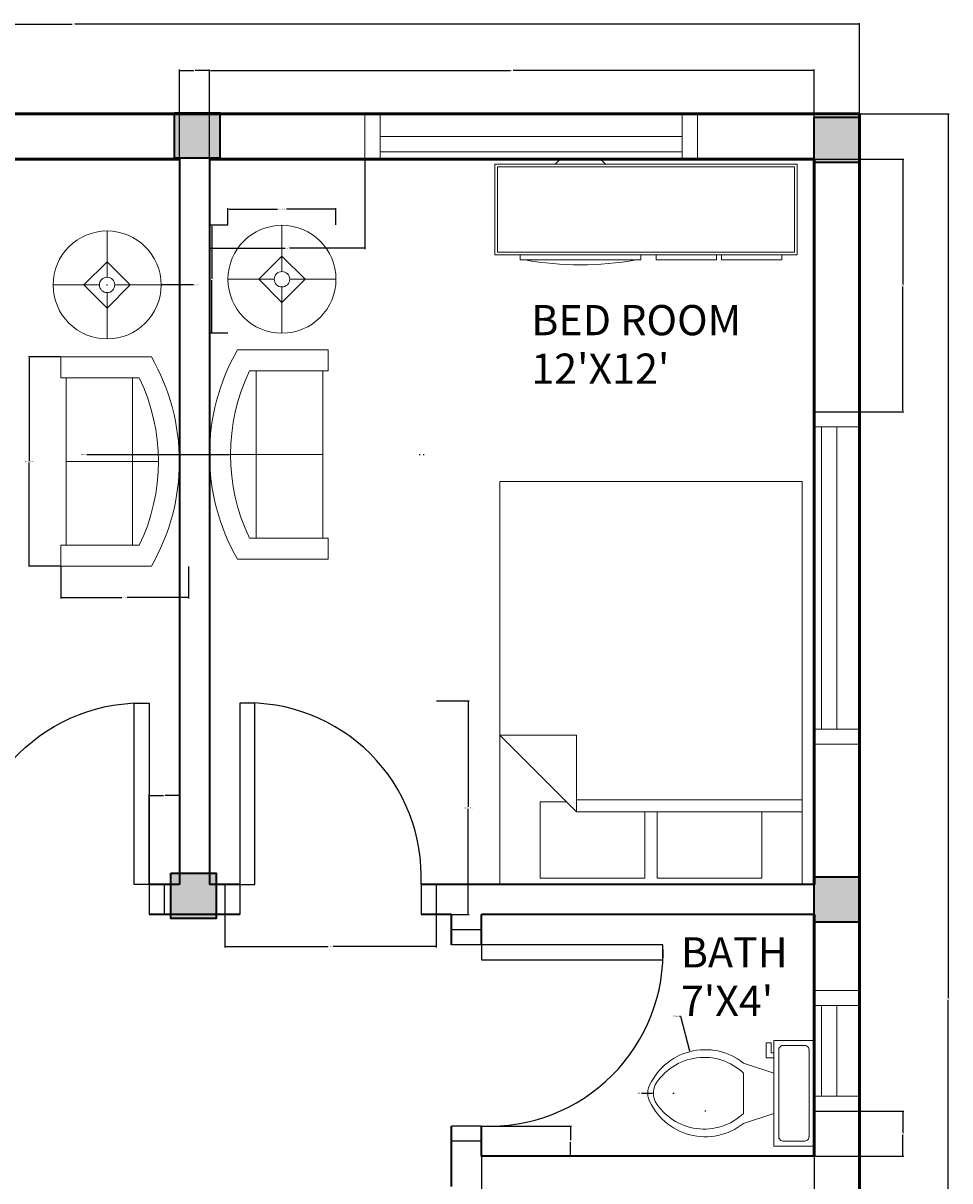
# Model space of a CAD drawing. Units: inches. Extents: x 2421 to 2780, y 382 to 769.
# Tile 4 of 4: x 2585 to 2769, y 539 to 769. Entities that reach past the tile are written whole.
import ezdxf

# ---------------------------------------------------------------- set-up
doc = ezdxf.new("R2010")
doc.units = ezdxf.units.IN
for name, color, linetype, lineweight in [('A-ANNO-DIMS', 2, 'Continuous', 18), ('A-AREA-IDEN', 7, 'Continuous', 25), ('A-COLS', 1, 'Continuous', 35), ('A-FLOR-FIXT', 3, 'Continuous', 18), ('DOOR', 1, 'Continuous', 25), ('FURNITURE', 3, 'Continuous', 18), ('INNER WALL', 2, 'Continuous', 35), ('OUTER WALL', 4, 'Continuous', 50), ('WINDOW', 5, 'Continuous', 18)]:
    doc.layers.add(name, color=color, linetype=linetype, lineweight=lineweight)
doc.styles.get("Standard").update_dxf_attribs({"font": 'arial.ttf'})
doc.dimstyles.get("Standard").update_dxf_attribs({"dimtxt": 0.18, "dimasz": 0.18, "dimexe": 0.18, "dimexo": 0.0625, "dimgap": 0.09, "dimtad": 0, "dimtih": 1, "dimtoh": 1, "dimdec": 4, "dimzin": 0, "dimdsep": 46, "dimtxsty": 'Standard', "dimcen": 0.09, "dimadec": 0, "dimazin": 0, "dimtfac": 1, "dimtdec": 4, "dimtofl": 0, "dimtmove": 0, "dimatfit": 3, "dimfxl": 1, "dimtolj": 1, "dimtzin": 0, "dimarcsym": 0})

# ---------------------------------------------------------------- blocks, each defined once
blk = doc.blocks.new('Toilet - top')
for p, q in [((9.5, -6), (9.5, -2)), ((-10, -8.5), (-8, -8.5)), ((-10, -9.5), (-10, -8.5)), ((-8, -8.5), (-8, -8)), ((-7, -8), (-7, -9.5)), ((-4, -8), (-6, -14)), ((4, -8), (6, -14)), ((-7, -9.5), (-10, -9.5)), ((4, -14), (-4, -14))]:
    blk.add_line(p, q)
blk.add_lwpolyline([(10.5, -8), (10.5, 0), (-10.5, 0), (-10.5, -8)], close=True)
for points in [[(-9.5, -2), (-9.5, -6)], [(8.5, -1), (-8.5, -1)], [(-8.5, -7), (8.5, -7)]]:
    blk.add_lwpolyline(points)
for centre, radius, start, end in [((-8.62, -1.88), 0.884, 81.8699, 188.1301), ((8.62, -1.88), 0.884, 351.8699, 98.1301), ((-8.62, -6.12), 0.884, 171.8699, 278.1301), ((8.62, -6.12), 0.884, 261.8699, 8.1301), ((3.52, -21.58), 12.17, 141.4691, 247.9714), ((4.2, -21.82), 11.33, 136.3677, 238.9468), ((-3.52, -21.58), 12.17, 292.0284, 38.5307), ((-4.2, -21.82), 11.33, 301.053, 43.6321), ((0, -27.88), 4, 245.7318, 294.2682), ((0, -29), 4, 254.8605, 285.1395)]:
    blk.add_arc(centre, radius, start, end)
blk = doc.blocks.new('Bed - Queen')
for p, q in [((0, -80.00003), (0, 0)), ((0, 0), (59.99999, 0)), ((59.99999, 0), (59.99999, -80.00003)), ((7.99999, -1.2), (28.79998, -1.2)), ((7.99999, -14.4), (7.99999, -1.2)), ((28.79998, -1.2), (28.79998, -14.4)), ((31.19999, -1.2), (51.99999, -1.2)), ((31.19999, -14.4), (31.19999, -1.2)), ((51.99999, -1.2), (51.99999, -16.4)), ((0, -14.4), (44.8, -14.4)), ((59.99999, -29.6), (44.8, -14.4)), ((44.8, -14.4), (44.8, -29.6)), ((44.8, -16.8), (0, -16.8)), ((51.99999, -16.4), (46.79936, -16.4)), ((44.8, -29.6), (59.99999, -29.6)), ((59.99999, -80.00003), (0, -80.00003))]:
    blk.add_line(p, q)
blk = doc.blocks.new('Sofa - Roundback Loveseat 5 ft.')
for p, q in [((0, -32.44198), (0, -5.99998)), ((-24, -33.99998), (-24, -11.46958)), ((24.00004, -33.99998), (24.00004, -11.46958)), ((-23.9998, -13.38178), (23.99986, -13.38178)), ((-24, -32.44198), (24.00004, -32.44198))]:
    blk.add_line(p, q)
for points in [[(-24, -33.99998), (-30, -33.99998), (-30, -7.99998)], [(30.00004, -7.99998), (30.00004, -33.99998), (24.00004, -33.99998)]]:
    blk.add_lwpolyline(points)
for centre, radius, start, end in [((0, -60.24998), 60.24998, 60.13715, 119.8628), ((0, -61.38438), 55.38444, 64.32083, 115.6792)]:
    blk.add_arc(centre, radius, start, end)
blk = doc.blocks.new('Lamp - Table')
for p, q in [((0, 7), (0, 1)), ((0, 3), (-3, 0)), ((3, 0), (0, 3)), ((-1, 0), (-7, 0)), ((-3, 0), (0, -3)), ((0, -3), (3, 0)), ((1, 0), (7, 0)), ((0, -1), (0, -7))]:
    blk.add_line(p, q)
for radius in [7, 1]:
    blk.add_circle((0, 0), radius)
blk = doc.blocks.new('Entertainment Center')
for p, q in [((-4, 0), (-5, -1)), ((4, 0), (-4, 0)), ((5, -1), (4, 0)), ((-17, -19), (-17, -1)), ((-17, -1), (43, -1)), ((-16.5, -18.5), (-16.5, -1.5)), ((-16.5, -1.5), (42.5, -1.5)), ((42.5, -1.5), (42.5, -18.5)), ((43, -1), (43, -19)), ((43, -19), (-17, -19)), ((42.5, -18.5), (-16.5, -18.5)), ((-12, -20), (-12, -19)), ((12, -20), (-12, -20)), ((12, -19), (12, -20)), ((15, -20), (15, -19)), ((27, -20), (15, -20)), ((27, -19), (27, -20)), ((28, -20), (28, -19)), ((40, -20), (28, -20)), ((40, -19), (40, -20))]:
    blk.add_line(p, q)
blk.add_arc((0, 40), 61, 259.6111, 280.3889)
blk = doc.blocks.new('DOOR-36IN-INT')
for p, q in [((0, 6), (0, 0)), ((3, 6), (3, 0)), ((39, 6), (39, 0)), ((42, 6), (42, 0))]:
    blk.add_line(p, q)
blk.add_lwpolyline([(3, 6), (6, 6), (6, 42), (3, 42)], close=True)
blk.add_arc((4.5, 7.5), 34.53, 357.5104, 92.4896)
blk = doc.blocks.new('WIN-60IN')
for p, q in [((0, 0), (0, 9)), ((3, 0), (3, 9)), ((63, 9), (63, 0)), ((66, 9), (66, 0)), ((63, 4.5), (3, 4.5)), ((63, 1.5), (3, 1.5))]:
    blk.add_line(p, q)
blk = doc.blocks.new('WIN-18IN')
for p, q in [((9, 24), (0, 24)), ((9, 21), (0, 21)), ((4.5, 21), (4.5, 3)), ((7.5, 21), (7.5, 3)), ((0, 3), (9, 3)), ((0, 0), (9, 0))]:
    blk.add_line(p, q)
blk = doc.blocks.new('COL-9X9IN')
h = blk.add_hatch(color=256)
h.dxf.hatch_style = 1
h.paths.add_polyline_path([(9, 9), (0, 9), (0, 0), (9, 0)])
blk.add_lwpolyline([(0, 9), (9, 9), (9, 0), (0, 0)], close=True)
blk = doc.blocks.new('*D24')
at = {"layer": 'A-ANNO-DIMS', "color": 0, "lineweight": -2, "transparency": 16777216}
for p, q in [((2667.53, 634.6), (2674.01, 634.6)), ((2673.83, 634.42), (2673.83, 613.57)), ((2673.83, 592.36), (2673.83, 613.21)), ((2667.53, 592.18), (2674.01, 592.18))]:
    blk.add_line(p, q, dxfattribs=at)
at = {"layer": 'A-ANNO-DIMS', "color": 0, "transparency": 16777216}
for points in [[(2673.8, 634.42), (2673.86, 634.42), (2673.83, 634.6)], [(2673.8, 592.36), (2673.86, 592.36), (2673.83, 592.18)]]:
    blk.add_solid(points, dxfattribs=at)
at = {"layer": 'Defpoints', "color": 0, "transparency": 16777216}
for p in [(2667.47, 634.6), (2673.83, 634.6), (2667.47, 592.18)]:
    blk.add_point(p, dxfattribs=at)
at = {"layer": 'A-ANNO-DIMS', "color": 0, "transparency": 16777216, "insert": (2673.83, 613.39), "char_height": 0.18, "attachment_point": 5}
blk.add_mtext('\\A1;DOOR 42 TYP.', dxfattribs=at)
blk = doc.blocks.new('*D25')
at = {"layer": 'A-ANNO-DIMS', "color": 0, "lineweight": -2, "transparency": 16777216}
for p, q in [((2625.47, 592.12), (2625.47, 585.64)), ((2667.47, 592.12), (2667.47, 585.64)), ((2625.65, 585.82), (2645.93, 585.82)), ((2667.29, 585.82), (2647, 585.82))]:
    blk.add_line(p, q, dxfattribs=at)
at = {"layer": 'A-ANNO-DIMS', "color": 0, "transparency": 16777216}
for points in [[(2625.65, 585.85), (2625.65, 585.79), (2625.47, 585.82)], [(2667.29, 585.85), (2667.29, 585.79), (2667.47, 585.82)]]:
    blk.add_solid(points, dxfattribs=at)
at = {"layer": 'Defpoints', "color": 0, "transparency": 16777216}
for p in [(2625.47, 592.18), (2667.47, 592.18), (2667.47, 585.82)]:
    blk.add_point(p, dxfattribs=at)
at = {"layer": 'A-ANNO-DIMS', "color": 0, "transparency": 16777216, "insert": (2646.47, 585.82), "char_height": 0.18, "attachment_point": 5}
blk.add_mtext('\\A1;42 TYP.', dxfattribs=at)
blk = doc.blocks.new('*D26')
at = {"layer": 'A-ANNO-DIMS', "color": 0, "lineweight": -2, "transparency": 16777216}
for p, q in [((2592.85, 702.92), (2586.5, 702.92)), ((2586.68, 702.74), (2586.68, 682.32)), ((2586.68, 661.54), (2586.68, 681.96)), ((2592.85, 661.36), (2586.5, 661.36))]:
    blk.add_line(p, q, dxfattribs=at)
at = {"layer": 'A-ANNO-DIMS', "color": 0, "transparency": 16777216}
for points in [[(2586.65, 702.74), (2586.71, 702.74), (2586.68, 702.92)], [(2586.65, 661.54), (2586.71, 661.54), (2586.68, 661.36)]]:
    blk.add_solid(points, dxfattribs=at)
at = {"layer": 'Defpoints', "color": 0, "transparency": 16777216}
for p in [(2592.91, 702.92), (2586.68, 661.36), (2592.91, 661.36)]:
    blk.add_point(p, dxfattribs=at)
at = {"layer": 'A-ANNO-DIMS', "color": 0, "transparency": 16777216, "insert": (2586.68, 682.14), "char_height": 0.18, "attachment_point": 5}
blk.add_mtext('\\A1;LOVESEAT 42 TYP.', dxfattribs=at)
blk = doc.blocks.new('*D27')
at = {"layer": 'A-ANNO-DIMS', "color": 0, "lineweight": -2, "transparency": 16777216}
for p, q in [((2592.91, 661.29), (2592.91, 654.94)), ((2618.31, 661.29), (2618.31, 654.94)), ((2593.09, 655.12), (2605.08, 655.12)), ((2618.13, 655.12), (2606.14, 655.12))]:
    blk.add_line(p, q, dxfattribs=at)
at = {"layer": 'A-ANNO-DIMS', "color": 0, "transparency": 16777216}
for points in [[(2593.09, 655.15), (2593.09, 655.09), (2592.91, 655.12)], [(2618.13, 655.15), (2618.13, 655.09), (2618.31, 655.12)]]:
    blk.add_solid(points, dxfattribs=at)
at = {"layer": 'Defpoints', "color": 0, "transparency": 16777216}
for p in [(2592.91, 661.36), (2618.31, 661.36), (2618.31, 655.12)]:
    blk.add_point(p, dxfattribs=at)
at = {"layer": 'A-ANNO-DIMS', "color": 0, "transparency": 16777216, "insert": (2605.61, 655.12), "char_height": 0.18, "attachment_point": 5}
blk.add_mtext('\\A1;25 TYP.', dxfattribs=at)
blk = doc.blocks.new('*D28')
at = {"layer": 'A-ANNO-DIMS', "color": 0, "lineweight": -2, "transparency": 16777216}
for p, q in [((2626.12, 729.13), (2626.12, 732.47)), ((2626.3, 732.29), (2635.94, 732.29)), ((2647.38, 732.29), (2637.74, 732.29)), ((2647.56, 729.13), (2647.56, 732.47))]:
    blk.add_line(p, q, dxfattribs=at)
at = {"layer": 'A-ANNO-DIMS', "color": 0, "transparency": 16777216}
for points in [[(2626.3, 732.32), (2626.3, 732.26), (2626.12, 732.29)], [(2647.38, 732.32), (2647.38, 732.26), (2647.56, 732.29)]]:
    blk.add_solid(points, dxfattribs=at)
at = {"layer": 'Defpoints', "color": 0, "transparency": 16777216}
for p in [(2647.56, 732.29), (2626.12, 729.07), (2647.56, 729.07)]:
    blk.add_point(p, dxfattribs=at)
at = {"layer": 'A-ANNO-DIMS', "color": 0, "transparency": 16777216, "insert": (2636.84, 732.29), "char_height": 0.18, "attachment_point": 5}
blk.add_mtext('\\A1;LAMP 21 TYP.', dxfattribs=at)
blk = doc.blocks.new('*D29')
at = {"layer": 'A-ANNO-DIMS', "color": 0, "lineweight": -2, "transparency": 16777216}
for p, q in [((2626.06, 729.07), (2622.72, 729.07)), ((2622.9, 728.89), (2622.9, 718.53)), ((2622.9, 707.81), (2622.9, 718.17)), ((2626.06, 707.63), (2622.72, 707.63))]:
    blk.add_line(p, q, dxfattribs=at)
at = {"layer": 'A-ANNO-DIMS', "color": 0, "transparency": 16777216}
for points in [[(2622.87, 728.89), (2622.93, 728.89), (2622.9, 729.07)], [(2622.87, 707.81), (2622.93, 707.81), (2622.9, 707.63)]]:
    blk.add_solid(points, dxfattribs=at)
at = {"layer": 'Defpoints', "color": 0, "transparency": 16777216}
for p in [(2622.9, 729.07), (2626.12, 729.07), (2626.12, 707.63)]:
    blk.add_point(p, dxfattribs=at)
at = {"layer": 'A-ANNO-DIMS', "color": 0, "transparency": 16777216, "insert": (2622.9, 718.35), "char_height": 0.18, "attachment_point": 5}
blk.add_mtext('\\A1;21 TYP.', dxfattribs=at)
blk = doc.blocks.new('*D46')
at = {"layer": 'A-ANNO-DIMS', "color": 0, "lineweight": -2, "transparency": 16777216}
for p, q in [((2439.47, 751.24), (2439.47, 769.21)), ((2439.65, 769.03), (2595.18, 769.03)), ((2751.29, 769.03), (2595.75, 769.03)), ((2751.47, 751.24), (2751.47, 769.21))]:
    blk.add_line(p, q, dxfattribs=at)
at = {"layer": 'A-ANNO-DIMS', "color": 0, "transparency": 16777216}
for points in [[(2439.65, 769.06), (2439.65, 769), (2439.47, 769.03)], [(2751.29, 769.06), (2751.29, 769), (2751.47, 769.03)]]:
    blk.add_solid(points, dxfattribs=at)
at = {"layer": 'Defpoints', "color": 0, "transparency": 16777216}
for p in [(2751.47, 769.03), (2439.47, 751.18), (2751.47, 751.18)]:
    blk.add_point(p, dxfattribs=at)
at = {"layer": 'A-ANNO-DIMS', "color": 0, "transparency": 16777216, "insert": (2595.47, 769.03), "char_height": 0.18, "attachment_point": 5}
blk.add_mtext('\\A1;312', dxfattribs=at)
blk = doc.blocks.new('*D47')
at = {"layer": 'A-ANNO-DIMS', "color": 0, "lineweight": -2, "transparency": 16777216}
for p, q in [((2751.53, 751.18), (2769.3, 751.18)), ((2769.12, 751), (2769.12, 575.56)), ((2769.12, 399.76), (2769.12, 575.2)), ((2664.93, 399.58), (2769.3, 399.58))]:
    blk.add_line(p, q, dxfattribs=at)
at = {"layer": 'A-ANNO-DIMS', "color": 0, "transparency": 16777216}
for points in [[(2769.09, 751), (2769.15, 751), (2769.12, 751.18)], [(2769.09, 399.76), (2769.15, 399.76), (2769.12, 399.58)]]:
    blk.add_solid(points, dxfattribs=at)
at = {"layer": 'Defpoints', "color": 0, "transparency": 16777216}
for p in [(2751.47, 751.18), (2664.86, 399.58), (2769.12, 399.58)]:
    blk.add_point(p, dxfattribs=at)
at = {"layer": 'A-ANNO-DIMS', "color": 0, "transparency": 16777216, "insert": (2769.12, 575.38), "char_height": 0.18, "attachment_point": 5}
blk.add_mtext('\\A1;351.6', dxfattribs=at)
blk = doc.blocks.new('*D52')
at = {"layer": 'A-ANNO-DIMS', "color": 0, "lineweight": -2, "transparency": 16777216}
for p, q in [((2622.47, 742.24), (2622.47, 760.01)), ((2622.65, 759.83), (2682.19, 759.83)), ((2742.29, 759.83), (2682.75, 759.83)), ((2742.47, 742.24), (2742.47, 760.01))]:
    blk.add_line(p, q, dxfattribs=at)
at = {"layer": 'A-ANNO-DIMS', "color": 0, "transparency": 16777216}
for points in [[(2622.65, 759.86), (2622.65, 759.8), (2622.47, 759.83)], [(2742.29, 759.86), (2742.29, 759.8), (2742.47, 759.83)]]:
    blk.add_solid(points, dxfattribs=at)
at = {"layer": 'Defpoints', "color": 0, "transparency": 16777216}
for p in [(2742.47, 759.83), (2622.47, 742.18), (2742.47, 742.18)]:
    blk.add_point(p, dxfattribs=at)
at = {"layer": 'A-ANNO-DIMS', "color": 0, "transparency": 16777216, "insert": (2682.47, 759.83), "char_height": 0.18, "attachment_point": 5}
blk.add_mtext('\\A1;120', dxfattribs=at)
blk = doc.blocks.new('*D53')
at = {"layer": 'A-ANNO-DIMS', "color": 0, "lineweight": -2, "transparency": 16777216}
for p, q in [((2676.47, 544.12), (2676.47, 526.35)), ((2742.47, 544.12), (2742.47, 526.35)), ((2676.65, 526.53), (2709.25, 526.53)), ((2742.29, 526.53), (2709.69, 526.53))]:
    blk.add_line(p, q, dxfattribs=at)
at = {"layer": 'A-ANNO-DIMS', "color": 0, "transparency": 16777216}
for points in [[(2676.65, 526.56), (2676.65, 526.5), (2676.47, 526.53)], [(2742.29, 526.56), (2742.29, 526.5), (2742.47, 526.53)]]:
    blk.add_solid(points, dxfattribs=at)
at = {"layer": 'Defpoints', "color": 0, "transparency": 16777216}
for p in [(2676.47, 544.18), (2742.47, 544.18), (2676.47, 526.53)]:
    blk.add_point(p, dxfattribs=at)
at = {"layer": 'A-ANNO-DIMS', "color": 0, "transparency": 16777216, "insert": (2709.47, 526.53), "char_height": 0.18, "attachment_point": 5}
blk.add_mtext('\\A1;66', dxfattribs=at)
blk = doc.blocks.new('*D55')
at = {"layer": 'A-ANNO-DIMS', "color": 0, "lineweight": -2, "transparency": 16777216}
for p, q in [((2616.47, 742.24), (2616.47, 760.01)), ((2616.65, 759.83), (2619.32, 759.83)), ((2622.29, 759.83), (2619.62, 759.83)), ((2622.47, 742.24), (2622.47, 760.01))]:
    blk.add_line(p, q, dxfattribs=at)
at = {"layer": 'A-ANNO-DIMS', "color": 0, "transparency": 16777216}
for points in [[(2616.65, 759.86), (2616.65, 759.8), (2616.47, 759.83)], [(2622.29, 759.86), (2622.29, 759.8), (2622.47, 759.83)]]:
    blk.add_solid(points, dxfattribs=at)
at = {"layer": 'Defpoints', "color": 0, "transparency": 16777216}
for p in [(2622.47, 759.83), (2616.47, 742.18), (2622.47, 742.18)]:
    blk.add_point(p, dxfattribs=at)
at = {"layer": 'A-ANNO-DIMS', "color": 0, "transparency": 16777216, "insert": (2619.47, 759.83), "char_height": 0.18, "attachment_point": 5}
blk.add_mtext('\\A1;6', dxfattribs=at)
blk = doc.blocks.new('*D57')
at = {"layer": 'A-ANNO-DIMS', "color": 0, "lineweight": -2, "transparency": 16777216}
for p, q in [((2622.47, 742.12), (2622.47, 724.35)), ((2653.31, 742.12), (2653.31, 724.35)), ((2622.65, 724.53), (2637.43, 724.53)), ((2653.13, 724.53), (2638.35, 724.53))]:
    blk.add_line(p, q, dxfattribs=at)
at = {"layer": 'A-ANNO-DIMS', "color": 0, "transparency": 16777216}
for points in [[(2622.65, 724.56), (2622.65, 724.5), (2622.47, 724.53)], [(2653.13, 724.56), (2653.13, 724.5), (2653.31, 724.53)]]:
    blk.add_solid(points, dxfattribs=at)
at = {"layer": 'Defpoints', "color": 0, "transparency": 16777216}
for p in [(2622.47, 742.18), (2653.31, 742.18), (2622.47, 724.53)]:
    blk.add_point(p, dxfattribs=at)
at = {"layer": 'A-ANNO-DIMS', "color": 0, "transparency": 16777216, "insert": (2637.89, 724.53), "char_height": 0.18, "attachment_point": 5}
blk.add_mtext('\\A1;30.846', dxfattribs=at)
blk = doc.blocks.new('*D58')
at = {"layer": 'A-ANNO-DIMS', "color": 0, "lineweight": -2, "transparency": 16777216}
for p, q in [((2742.53, 742.18), (2760.3, 742.18)), ((2760.12, 742), (2760.12, 717.29)), ((2760.12, 692.21), (2760.12, 716.92)), ((2742.53, 692.03), (2760.3, 692.03))]:
    blk.add_line(p, q, dxfattribs=at)
at = {"layer": 'A-ANNO-DIMS', "color": 0, "transparency": 16777216}
for points in [[(2760.09, 742), (2760.15, 742), (2760.12, 742.18)], [(2760.09, 692.21), (2760.15, 692.21), (2760.12, 692.03)]]:
    blk.add_solid(points, dxfattribs=at)
at = {"layer": 'Defpoints', "color": 0, "transparency": 16777216}
for p in [(2742.47, 742.18), (2742.47, 692.03), (2760.12, 692.03)]:
    blk.add_point(p, dxfattribs=at)
at = {"layer": 'A-ANNO-DIMS', "color": 0, "transparency": 16777216, "insert": (2760.12, 717.11), "char_height": 0.18, "attachment_point": 5}
blk.add_mtext('\\A1;50.15', dxfattribs=at)
blk = doc.blocks.new('*D62')
at = {"layer": 'A-ANNO-DIMS', "color": 0, "lineweight": -2, "transparency": 16777216}
for p, q in [((2742.53, 553.11), (2760.3, 553.11)), ((2760.12, 552.93), (2760.12, 548.83)), ((2760.12, 544.36), (2760.12, 548.46)), ((2742.53, 544.18), (2760.3, 544.18))]:
    blk.add_line(p, q, dxfattribs=at)
at = {"layer": 'A-ANNO-DIMS', "color": 0, "transparency": 16777216}
for points in [[(2760.09, 552.93), (2760.15, 552.93), (2760.12, 553.11)], [(2760.09, 544.36), (2760.15, 544.36), (2760.12, 544.18)]]:
    blk.add_solid(points, dxfattribs=at)
at = {"layer": 'Defpoints', "color": 0, "transparency": 16777216}
for p in [(2742.47, 553.11), (2742.47, 544.18), (2760.12, 544.18)]:
    blk.add_point(p, dxfattribs=at)
at = {"layer": 'A-ANNO-DIMS', "color": 0, "transparency": 16777216, "insert": (2760.12, 548.65), "char_height": 0.18, "attachment_point": 5}
blk.add_mtext('\\A1;8.93', dxfattribs=at)
blk = doc.blocks.new('*D68')
at = {"layer": 'A-ANNO-DIMS', "color": 0, "lineweight": -2, "transparency": 16777216}
for p, q in [((2610.47, 598.24), (2610.47, 616.01)), ((2610.65, 615.83), (2613.32, 615.83)), ((2616.29, 615.83), (2613.62, 615.83)), ((2616.47, 598.24), (2616.47, 616.01))]:
    blk.add_line(p, q, dxfattribs=at)
at = {"layer": 'A-ANNO-DIMS', "color": 0, "transparency": 16777216}
for points in [[(2610.65, 615.86), (2610.65, 615.8), (2610.47, 615.83)], [(2616.29, 615.86), (2616.29, 615.8), (2616.47, 615.83)]]:
    blk.add_solid(points, dxfattribs=at)
at = {"layer": 'Defpoints', "color": 0, "transparency": 16777216}
for p in [(2616.47, 615.83), (2610.47, 598.18), (2616.47, 598.18)]:
    blk.add_point(p, dxfattribs=at)
at = {"layer": 'A-ANNO-DIMS', "color": 0, "transparency": 16777216, "insert": (2613.47, 615.83), "char_height": 0.18, "attachment_point": 5}
blk.add_mtext('\\A1;6', dxfattribs=at)
blk = doc.blocks.new('*D70')
at = {"layer": 'A-ANNO-DIMS', "color": 0, "lineweight": -2, "transparency": 16777216}
for p, q in [((2676.53, 550.18), (2694.3, 550.18)), ((2694.12, 550), (2694.12, 547.36)), ((2694.12, 544.36), (2694.12, 547)), ((2676.53, 544.18), (2694.3, 544.18))]:
    blk.add_line(p, q, dxfattribs=at)
at = {"layer": 'A-ANNO-DIMS', "color": 0, "transparency": 16777216}
for points in [[(2694.09, 550), (2694.15, 550), (2694.12, 550.18)], [(2694.09, 544.36), (2694.15, 544.36), (2694.12, 544.18)]]:
    blk.add_solid(points, dxfattribs=at)
at = {"layer": 'Defpoints', "color": 0, "transparency": 16777216}
for p in [(2676.47, 550.18), (2676.47, 544.18), (2694.12, 544.18)]:
    blk.add_point(p, dxfattribs=at)
at = {"layer": 'A-ANNO-DIMS', "color": 0, "transparency": 16777216, "insert": (2694.12, 547.18), "char_height": 0.18, "attachment_point": 5}
blk.add_mtext('\\A1;6', dxfattribs=at)
blk = doc.blocks.new('*D77')
at = {"layer": 'A-ANNO-DIMS', "color": 0, "lineweight": -2, "transparency": 16777216}
for p, q in [((2598.1, 683.53), (2622.29, 683.53)), ((2664.11, 683.53), (2664.29, 683.53)), ((2664.2, 683.44), (2664.2, 683.62))]:
    blk.add_line(p, q, dxfattribs=at)
at = {"layer": 'A-ANNO-DIMS', "color": 0, "transparency": 16777216}
blk.add_solid([(2622.29, 683.56), (2622.29, 683.5), (2622.47, 683.53)], dxfattribs=at)
at = {"layer": 'Defpoints', "color": 0, "transparency": 16777216}
for p in [(2622.47, 683.53), (2664.2, 683.53)]:
    blk.add_point(p, dxfattribs=at)
at = {"layer": 'A-ANNO-DIMS', "color": 0, "transparency": 16777216, "insert": (2597.42, 683.53), "char_height": 0.18, "attachment_point": 5}
blk.add_mtext('\\A1;3X R41.74', dxfattribs=at)
blk = doc.blocks.new('*D78')
at = {"layer": 'A-ANNO-DIMS', "color": 0, "lineweight": -2, "transparency": 16777216}
for p, q in [((2604.35, 683.53), (2626.44, 683.53)), ((2664.9, 683.53), (2665.08, 683.53)), ((2664.99, 683.44), (2664.99, 683.62))]:
    blk.add_line(p, q, dxfattribs=at)
at = {"layer": 'A-ANNO-DIMS', "color": 0, "transparency": 16777216}
blk.add_solid([(2626.44, 683.56), (2626.44, 683.5), (2626.62, 683.53)], dxfattribs=at)
at = {"layer": 'Defpoints', "color": 0, "transparency": 16777216}
for p in [(2626.62, 683.53), (2664.99, 683.53)]:
    blk.add_point(p, dxfattribs=at)
at = {"layer": 'A-ANNO-DIMS', "color": 0, "transparency": 16777216, "insert": (2603.6, 683.53), "char_height": 0.18, "attachment_point": 5}
blk.add_mtext('\\A1;3X R38.366', dxfattribs=at)
blk = doc.blocks.new('*D79')
at = {"layer": 'A-ANNO-DIMS', "color": 0, "lineweight": -2, "transparency": 16777216}
for p, q in [((2715.76, 572.02), (2715.94, 572.02)), ((2715.94, 572.02), (2717.75, 565.13)), ((2720.8, 553.18), (2720.98, 553.18)), ((2720.89, 553.09), (2720.89, 553.27))]:
    blk.add_line(p, q, dxfattribs=at)
at = {"layer": 'A-ANNO-DIMS', "color": 0, "transparency": 16777216}
blk.add_solid([(2717.78, 565.14), (2717.72, 565.12), (2717.79, 564.95)], dxfattribs=at)
at = {"layer": 'Defpoints', "color": 0, "transparency": 16777216}
for p in [(2717.79, 564.95), (2720.89, 553.18)]:
    blk.add_point(p, dxfattribs=at)
at = {"layer": 'A-ANNO-DIMS', "color": 0, "transparency": 16777216, "insert": (2715.08, 572.02), "char_height": 0.18, "attachment_point": 5}
blk.add_mtext('\\A1;4X R12.17', dxfattribs=at)
blk = doc.blocks.new('*D81')
at = {"layer": 'A-ANNO-DIMS', "color": 0, "lineweight": -2, "transparency": 16777216}
for p, q in [((2708.19, 556.7), (2710.41, 556.7)), ((2714.5, 556.7), (2714.68, 556.7)), ((2714.59, 556.61), (2714.59, 556.79))]:
    blk.add_line(p, q, dxfattribs=at)
at = {"layer": 'A-ANNO-DIMS', "color": 0, "transparency": 16777216}
blk.add_solid([(2710.41, 556.73), (2710.41, 556.67), (2710.59, 556.7)], dxfattribs=at)
at = {"layer": 'Defpoints', "color": 0, "transparency": 16777216}
for p in [(2710.59, 556.7), (2714.59, 556.7)]:
    blk.add_point(p, dxfattribs=at)
at = {"layer": 'A-ANNO-DIMS', "color": 0, "transparency": 16777216, "insert": (2707.76, 556.7), "char_height": 0.18, "attachment_point": 5}
blk.add_mtext('\\A1;4X R4', dxfattribs=at)
blk = doc.blocks.new('*D82')
at = {"layer": 'A-ANNO-DIMS', "color": 0, "lineweight": -2, "transparency": 16777216}
for p, q in [((2602.12, 717.13), (2602.12, 717.31)), ((2602.03, 717.22), (2602.21, 717.22)), ((2619.28, 717.22), (2613.02, 717.22))]:
    blk.add_line(p, q, dxfattribs=at)
at = {"layer": 'A-ANNO-DIMS', "color": 0, "transparency": 16777216}
blk.add_solid([(2613.02, 717.25), (2613.02, 717.19), (2612.84, 717.22)], dxfattribs=at)
at = {"layer": 'Defpoints', "color": 0, "transparency": 16777216}
for p in [(2591.4, 717.22), (2612.84, 717.22)]:
    blk.add_point(p, dxfattribs=at)
at = {"layer": 'A-ANNO-DIMS', "color": 0, "transparency": 16777216, "insert": (2619.96, 717.22), "char_height": 0.18, "attachment_point": 5}
blk.add_mtext('\\A1;3X ∅21.44', dxfattribs=at)

msp = doc.modelspace()

# ---------------------------------------------------------------- linework, layer by layer
at = {"layer": 'INNER WALL'}
for p, q in [((2616.466, 742.1806), (2616.466, 598.1806)), ((2622.466, 742.1806), (2622.466, 598.1806)), ((2616.466, 598.1806), (2610.466, 598.1806)), ((2628.466, 598.1806), (2622.466, 598.1806)), ((2742.466, 598.1806), (2664.466, 598.1806)), ((2628.466, 592.1806), (2610.466, 592.1806)), ((2670.466, 592.1806), (2664.466, 592.1806)), ((2670.466, 592.1806), (2664.466, 592.1806)), ((2670.466, 586.1806), (2670.466, 592.1806)), ((2742.466, 592.1806), (2676.466, 592.1806)), ((2742.466, 592.1806), (2676.466, 592.1806)), ((2676.466, 586.1806), (2676.466, 592.1806)), ((2670.466, 538.1806), (2670.466, 550.1806)), ((2676.466, 544.1806), (2676.466, 550.1806)), ((2742.466, 544.1806), (2676.466, 544.1806))]:
    msp.add_line(p, q, dxfattribs=at)
at = {"layer": 'OUTER WALL'}
for p, q in [((2616.466, 742.1806), (2448.466, 742.1806)), ((2742.466, 742.1806), (2622.466, 742.1806)), ((2742.466, 598.1806), (2742.466, 742.1806)), ((2742.466, 544.1806), (2742.466, 592.1806))]:
    msp.add_line(p, q, dxfattribs=at)
msp.add_lwpolyline([(2656.7381, 439.1806), (2751.466, 439.1806), (2751.466, 751.1806), (2439.466, 751.1806), (2439.466, 439.1806), (2620.7381, 439.1806)], dxfattribs=at)

# ---------------------------------------------------------------- block references
at = {"layer": 'A-COLS'}
for p in [(2615.5287, 742.3757), (2742.466, 741.507), (2614.7542, 591.3868), (2742.466, 590.6806)]:
    msp.add_blockref('COL-9X9IN', p, dxfattribs=at)
at = {"layer": 'A-FLOR-FIXT', "rotation": 270}
msp.add_blockref('Toilet - top', (2742.466, 556.704), dxfattribs=at)
at = {"layer": 'DOOR', "extrusion": (0, 0, -1), "zscale": -1}
msp.add_blockref('DOOR-36IN-INT', (-2613.466, 592.1806), dxfattribs=at)
at = {"layer": 'DOOR'}
msp.add_blockref('DOOR-36IN-INT', (2625.466, 592.1806), dxfattribs=at)
at = {"layer": 'DOOR', "rotation": 269.9999999999991}
msp.add_blockref('DOOR-36IN-INT', (2670.466, 589.1806), dxfattribs=at)
at = {"layer": 'FURNITURE'}
msp.add_blockref('Entertainment Center', (2696.098, 742.2028), dxfattribs=at)
at = {"layer": 'FURNITURE', "xscale": 1.531444562550245, "yscale": 1.531444562550245, "zscale": 1.531444562550245}
for p in [(2636.84, 718.3506), (2602.1243, 717.2195)]:
    msp.add_blockref('Lamp - Table', p, dxfattribs=at)
at = {"layer": 'FURNITURE', "xscale": 0.6927207335329854, "yscale": 0.6927207335329854, "zscale": 0.6927207335329854}
for p, rotation in [((2622.466, 683.531), 90), ((2616.466, 682.1386), 270)]:
    msp.add_blockref('Sofa - Roundback Loveseat 5 ft.', p, dxfattribs=dict(at, rotation=rotation))
at = {"layer": 'FURNITURE', "rotation": 180}
msp.add_blockref('Bed - Queen', (2740.0906, 598.1806), dxfattribs=at)
at = {"layer": 'WINDOW'}
msp.add_blockref('WIN-60IN', (2653.3125, 742.1806), dxfattribs=at)
for name, p, rotation in [('WIN-60IN', (2742.466, 692.0305), 269.9999999999999), ('WIN-18IN', (2751.466, 577.1114), 180)]:
    msp.add_blockref(name, p, dxfattribs=dict(at, rotation=rotation))

# ---------------------------------------------------------------- texts
at = {"layer": 'A-AREA-IDEN'}
for s, p in [('BED ROOM', (2686.3376, 707.2294)), ("12'X12'", (2686.3376, 697.5909)), ('BATH', (2716.0312, 581.6806)), ("7'X4'", (2716.0312, 572.0422))]:
    msp.add_text(s, height=6, dxfattribs=at).set_placement(p)

# ---------------------------------------------------------------- dimensions: what is measured, and where the dimension line sits
at = {"layer": 'A-ANNO-DIMS'}
for base, p1, p2, picture, middle in [((2751.466, 769.0257), (2439.466, 751.1806), (2751.466, 751.1806), '*D46', (2595.466, 769.0257)), ((2622.466, 759.8306), (2616.466, 742.1806), (2622.466, 742.1806), '*D55', (2619.466, 759.8306)), ((2742.466, 759.8306), (2622.466, 742.1806), (2742.466, 742.1806), '*D52', (2682.466, 759.8306)), ((2616.466, 615.8306), (2610.466, 598.1806), (2616.466, 598.1806), '*D68', (2613.466, 615.8306))]:
    dim = msp.add_linear_dim(base=base, p1=p1, p2=p2, dimstyle='Standard', override={"dimdec": 0, "dimlfac": 1, "dimrnd": 0, "dimzin": 0, "dimdsep": 46, "dimlunit": 2}, dxfattribs=at)
    dim.commit()
    dim.dimension.update_dxf_attribs({"geometry": picture, "text_midpoint": middle})
for base, p1, p2, angle, override, picture, middle in [((2769.116, 399.5831), (2751.466, 751.1806), (2664.8646, 399.5831), 90, {"dimdec": 1, "dimlfac": 1, "dimrnd": 0, "dimzin": 0, "dimdsep": 46, "dimlunit": 2}, '*D47', (2769.116, 575.3818)), ((2622.46599, 724.53057), (2653.31248, 742.18057), (2622.46599, 742.18057), 180, {"dimdec": 3, "dimlfac": 1, "dimrnd": 0, "dimzin": 0, "dimdsep": 46, "dimlunit": 2}, '*D57', (2637.88924, 724.53057)), ((2760.116, 692.0305), (2742.466, 742.1806), (2742.466, 692.0305), 270, {"dimdec": 2, "dimlfac": 1, "dimrnd": 0, "dimzin": 0, "dimdsep": 46, "dimlunit": 2}, '*D58', (2760.116, 717.1055)), ((2760.116, 544.1806), (2742.466, 553.1114), (2742.466, 544.1806), 270, {"dimdec": 2, "dimlfac": 1, "dimrnd": 0, "dimzin": 0, "dimdsep": 46, "dimlunit": 2}, '*D62', (2760.116, 548.646)), ((2694.116, 544.1806), (2676.466, 550.1806), (2676.466, 544.1806), 270, {"dimdec": 0, "dimlfac": 1, "dimrnd": 0, "dimzin": 0, "dimdsep": 46, "dimlunit": 2}, '*D70', (2694.116, 547.1806)), ((2676.466, 526.5306), (2742.466, 544.1806), (2676.466, 544.1806), 180, {"dimdec": 0, "dimlfac": 1, "dimrnd": 0, "dimzin": 0, "dimdsep": 46, "dimlunit": 2}, '*D53', (2709.466, 526.5306))]:
    dim = msp.add_linear_dim(base=base, p1=p1, p2=p2, angle=angle, dimstyle='Standard', override=override, dxfattribs=at)
    dim.commit()
    dim.dimension.update_dxf_attribs({"geometry": picture, "text_midpoint": middle})
for base, p1, p2, text, picture, middle in [((2647.5601, 732.2868), (2626.1199, 729.0707), (2647.5601, 729.0707), 'LAMP <> TYP.', '*D28', (2636.84, 732.2868)), ((2618.3132, 655.1225), (2592.9135, 661.357), (2618.3132, 661.357), '<> TYP.', '*D27', (2605.6134, 655.1225)), ((2667.466, 585.8175), (2625.466, 592.1806), (2667.466, 592.1806), '<> TYP.', '*D25', (2646.466, 585.8175))]:
    dim = msp.add_linear_dim(base=base, p1=p1, p2=p2, text=text, dimstyle='Standard', override={"dimdec": 0, "dimlfac": 1, "dimrnd": 0, "dimzin": 0, "dimdsep": 46, "dimlunit": 2}, dxfattribs=at)
    dim.commit()
    dim.dimension.update_dxf_attribs({"geometry": picture, "text_midpoint": middle})
for base, p1, p2, angle, text, picture, middle in [((2622.9039, 729.0707), (2626.1199, 707.6305), (2626.1199, 729.0707), 90, '<> TYP.', '*D29', (2622.9039, 718.3506)), ((2586.679, 661.357), (2592.9135, 702.9202), (2592.9135, 661.357), 270, 'LOVESEAT <> TYP.', '*D26', (2586.679, 682.1386)), ((2673.8291, 634.601), (2667.466, 592.1806), (2667.466, 634.601), 90, 'DOOR <> TYP.', '*D24', (2673.8291, 613.3908))]:
    dim = msp.add_linear_dim(base=base, p1=p1, p2=p2, angle=angle, text=text, dimstyle='Standard', override={"dimdec": 0, "dimlfac": 1, "dimrnd": 0, "dimzin": 0, "dimdsep": 46, "dimlunit": 2}, dxfattribs=at)
    dim.commit()
    dim.dimension.update_dxf_attribs({"geometry": picture, "text_midpoint": middle})
dim = msp.add_diameter_dim_2p(p1=(2591.4041, 717.22), p2=(2612.8444, 717.219), text='3X <>', dimstyle='Standard', override={"dimdec": 2, "dimlfac": 1, "dimrnd": 0, "dimzin": 0, "dimdsep": 46, "dimlunit": 2}, dxfattribs=at)
dim.commit()
dim.dimension.update_dxf_attribs({"geometry": '*D82', "text_midpoint": (2619.2764, 717.2187), "dimtype": 163})
for center, mpoint, text, override, picture, middle in [((2664.2024, 683.531), (2622.466, 683.531), '3X <>', {"dimdec": 2, "dimlfac": 1, "dimrnd": 0, "dimzin": 0, "dimdsep": 46, "dimlunit": 2}, '*D77', (2597.4241, 683.531)), ((2664.9882, 683.531), (2626.6223, 683.531), '3X <>', {"dimdec": 3, "dimlfac": 1, "dimrnd": 0, "dimzin": 0, "dimdsep": 46, "dimlunit": 2}, '*D78', (2603.6027, 683.531)), ((2720.8855, 553.1844), (2717.793, 564.954), '4X <>', {"dimdec": 2, "dimlfac": 1, "dimrnd": 0, "dimzin": 0, "dimdsep": 46, "dimlunit": 2}, '*D79', (2715.0807, 572.0157)), ((2714.5895, 556.704), (2710.5895, 556.704), '4X <>', {"dimdec": 0, "dimlfac": 1, "dimrnd": 0, "dimzin": 0, "dimdsep": 46, "dimlunit": 2}, '*D81', (2708.1895, 556.704))]:
    dim = msp.add_radius_dim(center=center, mpoint=mpoint, text=text, dimstyle='Standard', override=override, dxfattribs=at)
    dim.commit()
    dim.dimension.update_dxf_attribs({"geometry": picture, "text_midpoint": middle, "dimtype": 164})

doc.saveas('drawing.dxf')
